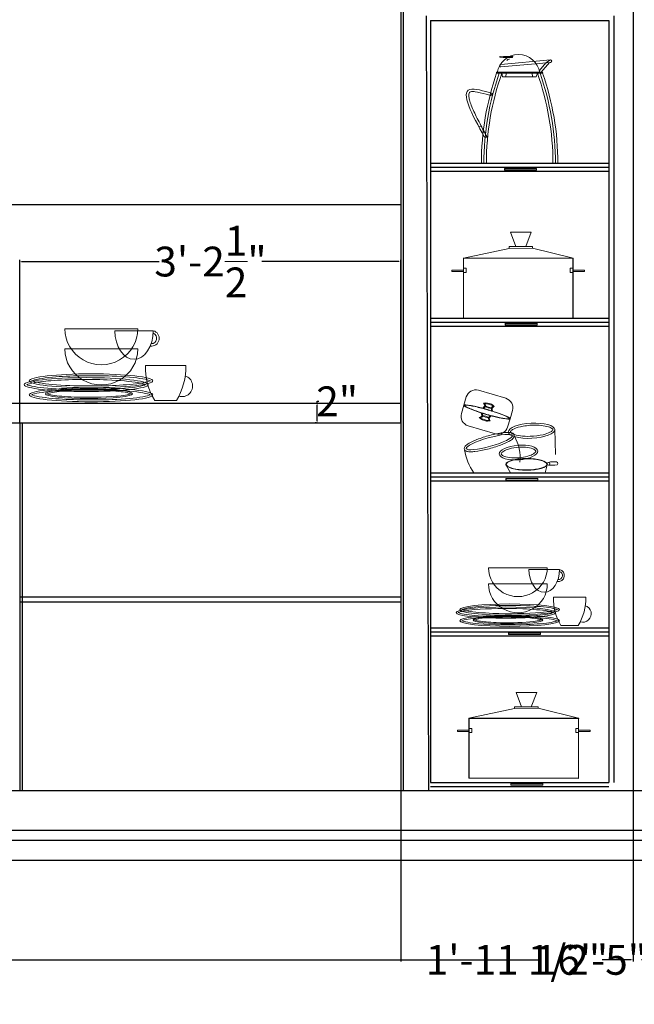
# Model space of a CAD drawing. Units: inches. Extents: x 1686244 to 1686928, y 1936095 to 1936489.
# Tile 3 of 11: x 1686303 to 1686365, y 1936336 to 1936435. Entities that reach past the tile are written whole.
import ezdxf

# ---------------------------------------------------------------- set-up
doc = ezdxf.new("R2010")
doc.units = ezdxf.units.IN
doc.header["$MEASUREMENT"] = 0
for name, color, linetype, lineweight in [('A-ANNO-DIMS', 240, 'Continuous', 18), ('A-ELEV', 7, 'Continuous', 25), ('A-FURN', 40, 'Continuous', 18)]:
    doc.layers.add(name, color=color, linetype=linetype, lineweight=lineweight)
doc.styles.get("Standard").update_dxf_attribs({"font": 'arial.ttf'})
doc.dimstyles.get("Standard").update_dxf_attribs({"dimtxt": 3, "dimasz": 0.18, "dimexe": 0.18, "dimexo": 0.0625, "dimgap": 0.09, "dimtad": 0, "dimtih": 1, "dimtoh": 1, "dimzin": 0, "dimdsep": 46, "dimlunit": 4, "dimtxsty": 'Standard', "dimcen": 0.09, "dimadec": 0, "dimazin": 0, "dimtfac": 1, "dimtofl": 0, "dimtmove": 0, "dimatfit": 3, "dimfxl": 1, "dimtolj": 1, "dimtzin": 0, "dimarcsym": 0})

# ---------------------------------------------------------------- blocks, each defined once
blk = doc.blocks.new('*D4')
at = {"layer": 'A-ANNO-DIMS', "color": 0, "lineweight": -2, "transparency": 16777216}
for p, q in [((1686303.305, 1936394.476), (1686303.305, 1936410.845)), ((1686303.485, 1936410.665), (1686317.355, 1936410.665)), ((1686341.513, 1936410.665), (1686327.696, 1936410.665)), ((1686341.693, 1936394.476), (1686341.693, 1936410.845))]:
    blk.add_line(p, q, dxfattribs=at)
at = {"layer": 'A-ANNO-DIMS', "color": 0, "transparency": 16777216}
for points in [[(1686303.485, 1936410.695), (1686303.485, 1936410.635), (1686303.305, 1936410.665)], [(1686341.513, 1936410.695), (1686341.513, 1936410.635), (1686341.693, 1936410.665)]]:
    blk.add_solid(points, dxfattribs=at)
at = {"layer": 'Defpoints', "color": 0, "transparency": 16777216}
for p in [(1686341.693, 1936410.665), (1686303.305, 1936394.414), (1686341.693, 1936394.414)]:
    blk.add_point(p, dxfattribs=at)
at = {"layer": 'A-ANNO-DIMS', "color": 0, "transparency": 16777216, "insert": (1686322.526, 1936410.665), "char_height": 3, "attachment_point": 5}
blk.add_mtext('\\A1;3\'-2{\\H1x;\\S1/2;}"', dxfattribs=at)
blk = doc.blocks.new('*D56')
at = {"layer": 'A-ANNO-DIMS', "color": 0, "lineweight": -2, "transparency": 16777216}
for p, q in [((1686333.27, 1936396.414), (1686333.27, 1936396.594)), ((1686333.27, 1936396.594), (1686333.45, 1936396.594)), ((1686333.27, 1936394.594), (1686333.27, 1936396.234)), ((1686333.333, 1936396.414), (1686333.45, 1936396.414)), ((1686333.208, 1936394.414), (1686333.09, 1936394.414))]:
    blk.add_line(p, q, dxfattribs=at)
at = {"layer": 'A-ANNO-DIMS', "color": 0, "transparency": 16777216}
for points in [[(1686333.24, 1936396.234), (1686333.3, 1936396.234), (1686333.27, 1936396.414)], [(1686333.24, 1936394.594), (1686333.3, 1936394.594), (1686333.27, 1936394.414)]]:
    blk.add_solid(points, dxfattribs=at)
at = {"layer": 'Defpoints', "color": 0, "transparency": 16777216}
for p in [(1686333.27, 1936396.414), (1686333.27, 1936396.414), (1686333.27, 1936394.414)]:
    blk.add_point(p, dxfattribs=at)
at = {"layer": 'A-ANNO-DIMS', "color": 0, "transparency": 16777216, "insert": (1686335.29, 1936396.594), "char_height": 3, "attachment_point": 5}
blk.add_mtext('\\A1;2"', dxfattribs=at)
blk = doc.blocks.new('COOKING-POT')
for p, q in [((0.009, 6.061), (4.609, 7.038)), ((4.609, 7.038), (4.609, 7.206)), ((4.609, 7.038), (6.983, 7.07)), ((4.629, 7.226), (6.962, 7.226)), ((6.982, 7.206), (6.983, 7.07)), ((11.059, 6.061), (6.983, 7.07)), ((0.029, 6.041), (0.009, 6.041)), ((11.039, 6.041), (11.059, 6.041))]:
    blk.add_line(p, q)
for points in [[(11.059, 6.061), (0.009, 6.061)], [(0.009, 0.022), (11.059, 0), (11.059, 6.041)], [(0.009, 6.041), (0.009, 0.022)]]:
    blk.add_lwpolyline(points)
blk.add_lwpolyline([(0.029, 0.042), (11.039, 0.022), (11.039, 6.041), (0.029, 6.041)], close=True)
for centre, radius, start, end in [((4.629, 7.206), 0.0201, 90, 180), ((6.962, 7.206), 0.0201, 0.77462, 90), ((0.01, 6.051), 0.0101, 93.59862, 266.40138), ((11.058, 6.051), 0.0101, 273.59862, 86.40138)]:
    blk.add_arc(centre, radius, start, end)
blk = doc.blocks.new('*D87')
at = {"layer": 'A-ANNO-DIMS', "color": 0, "lineweight": -2, "transparency": 16777216}
for p, q in [((1686262.353, 1936350.349), (1686262.353, 1936340.182)), ((1686459.353, 1936350.349), (1686459.353, 1936340.182)), ((1686262.533, 1936340.362), (1686355.751, 1936340.362)), ((1686459.173, 1936340.362), (1686365.954, 1936340.362))]:
    blk.add_line(p, q, dxfattribs=at)
at = {"layer": 'A-ANNO-DIMS', "color": 0, "transparency": 16777216}
for points in [[(1686262.533, 1936340.392), (1686262.533, 1936340.332), (1686262.353, 1936340.362)], [(1686459.173, 1936340.392), (1686459.173, 1936340.332), (1686459.353, 1936340.362)]]:
    blk.add_solid(points, dxfattribs=at)
at = {"layer": 'Defpoints', "color": 0, "transparency": 16777216}
for p in [(1686262.353, 1936350.412), (1686459.353, 1936350.412), (1686459.353, 1936340.362)]:
    blk.add_point(p, dxfattribs=at)
at = {"layer": 'A-ANNO-DIMS', "color": 0, "transparency": 16777216, "insert": (1686360.853, 1936340.362), "char_height": 3, "attachment_point": 5}
blk.add_mtext('\\A1;16\'-5"', dxfattribs=at)
blk = doc.blocks.new('*D90')
at = {"layer": 'A-ANNO-DIMS', "color": 0, "lineweight": -2, "transparency": 16777216}
for p, q in [((1686341.693, 1936357.349), (1686341.693, 1936340.182)), ((1686365.103, 1936357.349), (1686365.103, 1936340.182)), ((1686341.873, 1936340.362), (1686344.801, 1936340.362)), ((1686364.923, 1936340.362), (1686361.995, 1936340.362))]:
    blk.add_line(p, q, dxfattribs=at)
at = {"layer": 'A-ANNO-DIMS', "color": 0, "transparency": 16777216}
for points in [[(1686341.873, 1936340.392), (1686341.873, 1936340.332), (1686341.693, 1936340.362)], [(1686364.923, 1936340.392), (1686364.923, 1936340.332), (1686365.103, 1936340.362)]]:
    blk.add_solid(points, dxfattribs=at)
at = {"layer": 'Defpoints', "color": 0, "transparency": 16777216}
for p in [(1686341.693, 1936357.412), (1686365.103, 1936357.412), (1686365.103, 1936340.362)]:
    blk.add_point(p, dxfattribs=at)
at = {"layer": 'A-ANNO-DIMS', "color": 0, "transparency": 16777216, "insert": (1686353.398, 1936340.362), "char_height": 3, "attachment_point": 5}
blk.add_mtext('\\A1;1\'-11 1/2"', dxfattribs=at)

msp = doc.modelspace()

# ---------------------------------------------------------------- linework, layer by layer
at = {"layer": 'A-ELEV'}
for p, q in [((1686341.693, 1936467.412), (1686341.693, 1936357.412)), ((1686341.943, 1936467.412), (1686341.943, 1936357.412)), ((1686365.103, 1936467.412), (1686365.103, 1936357.412)), ((1686344.26, 1936435.412), (1686344.495, 1936357.412)), ((1686363.15, 1936435.412), (1686363.15, 1936358.215)), ((1686344.7, 1936434.948), (1686344.7, 1936358.215)), ((1686344.7, 1936434.948), (1686362.65, 1936434.948)), ((1686362.65, 1936434.948), (1686362.65, 1936358.215)), ((1686344.7, 1936420.566), (1686362.65, 1936420.566)), ((1686344.7, 1936420.164), (1686362.65, 1936420.164)), ((1686344.7, 1936419.762), (1686362.65, 1936419.762)), ((1686262.353, 1936416.412), (1686341.693, 1936416.412)), ((1686344.7, 1936404.978), (1686362.65, 1936404.978)), ((1686344.7, 1936404.576), (1686362.65, 1936404.576)), ((1686344.7, 1936404.175), (1686362.65, 1936404.175)), ((1686262.353, 1936396.412), (1686341.687, 1936396.414)), ((1686262.353, 1936394.412), (1686341.693, 1936394.414)), ((1686303.305, 1936394.414), (1686303.305, 1936357.414)), ((1686303.555, 1936394.414), (1686303.555, 1936357.414)), ((1686344.7, 1936389.391), (1686362.65, 1936389.391)), ((1686344.7, 1936388.989), (1686362.65, 1936388.989)), ((1686344.7, 1936388.587), (1686362.65, 1936388.587)), ((1686303.305, 1936376.914), (1686341.746, 1936376.914)), ((1686303.305, 1936376.414), (1686341.748, 1936376.414)), ((1686344.7, 1936373.803), (1686362.65, 1936373.803)), ((1686344.7, 1936373.401), (1686362.65, 1936373.401)), ((1686344.7, 1936372.999), (1686362.65, 1936372.999)), ((1686344.7, 1936358.215), (1686362.65, 1936358.215)), ((1686343.995, 1936357.412), (1686343.995, 1936357.41)), ((1686344.222, 1936357.412), (1686362.975, 1936357.412)), ((1686344.7, 1936357.814), (1686362.65, 1936357.814)), ((1686262.353, 1936353.412), (1686459.353, 1936353.412)), ((1686262.353, 1936352.412), (1686459.353, 1936352.412)), ((1686262.353, 1936350.412), (1686459.353, 1936350.412))]:
    msp.add_line(p, q, dxfattribs=at)
msp.add_lwpolyline([(1686459.353, 1936357.412), (1686459.353, 1936467.412), (1686262.353, 1936467.412), (1686262.353, 1936357.412)], close=True, dxfattribs=at)
at = {"layer": 'A-FURN'}
for p, q in [((1686351.713, 1936431.294), (1686352.069, 1936431.279)), ((1686352.084, 1936431.298), (1686352.011, 1936431.201)), ((1686352.992, 1936431.298), (1686352.084, 1936431.298)), ((1686352.969, 1936431.201), (1686352.992, 1936431.298)), ((1686352.048, 1936431.249), (1686351.685, 1936431.249)), ((1686351.763, 1936430.503), (1686356.77, 1936430.959)), ((1686351.786, 1936430.255), (1686356.793, 1936430.711)), ((1686352.011, 1936431.201), (1686352.969, 1936431.201)), ((1686356.327, 1936430.669), (1686355.661, 1936429.9)), ((1686356.684, 1936430.701), (1686355.831, 1936429.716)), ((1686356.782, 1936430.96), (1686356.327, 1936430.669)), ((1686351.359, 1936429.678), (1686351.359, 1936429.716)), ((1686351.359, 1936429.716), (1686355.991, 1936429.716)), ((1686351.359, 1936429.678), (1686355.991, 1936429.678)), ((1686351.359, 1936429.629), (1686355.991, 1936429.629)), ((1686351.886, 1936429.629), (1686351.955, 1936429.258)), ((1686352.328, 1936429.629), (1686352.277, 1936429.258)), ((1686354.895, 1936429.629), (1686355.006, 1936429.258)), ((1686355.331, 1936429.258), (1686355.464, 1936429.629)), ((1686355.991, 1936429.716), (1686355.991, 1936429.678)), ((1686351.955, 1936429.258), (1686355.331, 1936429.258)), ((1686350.957, 1936427.571), (1686350.765, 1936427.369)), ((1686349.549, 1936424.256), (1686349.803, 1936424.307)), ((1686350.408, 1936423.194), (1686350.127, 1936423.189)), ((1686349.821, 1936420.571), (1686357.528, 1936420.571)), ((1686349.821, 1936420.566), (1686357.528, 1936420.566)), ((1686353.3, 1936412.182), (1686352.753, 1936413.613)), ((1686352.753, 1936413.613), (1686354.833, 1936413.613)), ((1686354.286, 1936412.182), (1686354.833, 1936413.613)), ((1686348.007, 1936409.808), (1686346.848, 1936409.808)), ((1686346.848, 1936409.808), (1686346.848, 1936409.674)), ((1686346.848, 1936409.674), (1686348.007, 1936409.674)), ((1686348.007, 1936409.674), (1686348.007, 1936409.808)), ((1686359.057, 1936409.808), (1686360.216, 1936409.808)), ((1686359.057, 1936409.674), (1686359.057, 1936409.808)), ((1686360.216, 1936409.674), (1686359.057, 1936409.674)), ((1686360.216, 1936409.808), (1686360.216, 1936409.674)), ((1686307.855, 1936403.901), (1686315.213, 1936403.901)), ((1686312.902, 1936403.697), (1686316.76, 1936403.697)), ((1686307.855, 1936401.868), (1686315.213, 1936401.868)), ((1686315.975, 1936400.215), (1686320.037, 1936400.215)), ((1686316.918, 1936396.663), (1686319.094, 1936396.663)), ((1686357.217, 1936393.798), (1686357.274, 1936391.243)), ((1686352.366, 1936390.092), (1686352.754, 1936389.402)), ((1686356.251, 1936389.379), (1686356.451, 1936390.209)), ((1686352.754, 1936389.402), (1686356.251, 1936389.379)), ((1686350.548, 1936379.844), (1686356.46, 1936379.844)), ((1686354.603, 1936379.679), (1686357.703, 1936379.679)), ((1686350.548, 1936378.21), (1686356.46, 1936378.21)), ((1686357.072, 1936376.882), (1686360.336, 1936376.882)), ((1686357.83, 1936374.028), (1686359.578, 1936374.028)), ((1686353.862, 1936365.849), (1686353.315, 1936367.281)), ((1686353.315, 1936367.281), (1686355.395, 1936367.281)), ((1686354.848, 1936365.849), (1686355.395, 1936367.281)), ((1686348.569, 1936363.476), (1686347.41, 1936363.476)), ((1686347.41, 1936363.476), (1686347.41, 1936363.342)), ((1686347.41, 1936363.342), (1686348.569, 1936363.342)), ((1686348.569, 1936363.342), (1686348.569, 1936363.476)), ((1686359.619, 1936363.476), (1686360.778, 1936363.476)), ((1686359.619, 1936363.342), (1686359.619, 1936363.476)), ((1686360.778, 1936363.342), (1686359.619, 1936363.342)), ((1686360.778, 1936363.476), (1686360.778, 1936363.342))]:
    msp.add_line(p, q, dxfattribs=at)
for points in [[(1686352.147, 1936420.033), (1686355.381, 1936420.034), (1686355.381, 1936419.857), (1686352.147, 1936419.855)], [(1686352.167, 1936420.013), (1686355.361, 1936420.014), (1686355.361, 1936419.877), (1686352.167, 1936419.875)], [(1686348.3, 1936409.992), (1686348.027, 1936409.992), (1686348.027, 1936409.569), (1686348.3, 1936409.569)], [(1686358.764, 1936409.992), (1686359.037, 1936409.992), (1686359.037, 1936409.569), (1686358.764, 1936409.569)], [(1686352.219, 1936404.452), (1686355.454, 1936404.454), (1686355.454, 1936404.276), (1686352.219, 1936404.275)], [(1686352.239, 1936404.432), (1686355.434, 1936404.434), (1686355.434, 1936404.296), (1686352.239, 1936404.295)], [(1686352.29, 1936388.829), (1686355.524, 1936388.83), (1686355.524, 1936388.653), (1686352.29, 1936388.651)], [(1686352.31, 1936388.809), (1686355.504, 1936388.81), (1686355.504, 1936388.673), (1686352.31, 1936388.672)], [(1686352.553, 1936373.301), (1686355.787, 1936373.303), (1686355.787, 1936373.125), (1686352.553, 1936373.124)], [(1686352.573, 1936373.281), (1686355.767, 1936373.282), (1686355.767, 1936373.145), (1686352.573, 1936373.144)], [(1686348.862, 1936363.659), (1686348.589, 1936363.659), (1686348.589, 1936363.237), (1686348.862, 1936363.237)], [(1686359.326, 1936363.659), (1686359.599, 1936363.659), (1686359.599, 1936363.237), (1686359.326, 1936363.237)], [(1686352.781, 1936358.12), (1686356.016, 1936358.121), (1686356.016, 1936357.944), (1686352.781, 1936357.942)], [(1686352.801, 1936358.1), (1686355.996, 1936358.101), (1686355.996, 1936357.964), (1686352.801, 1936357.962)]]:
    msp.add_lwpolyline(points, close=True, dxfattribs=at)
for points in [[(1686348.054, 1936396.197), (1686348.3, 1936397.036, -0.414214), (1686349.522, 1936397.705), (1686352.284, 1936396.896, -0.414214), (1686352.953, 1936395.674), (1686352.707, 1936394.835)], [(1686348.054, 1936396.197), (1686347.808, 1936395.358, 0.414214), (1686348.477, 1936394.136), (1686351.239, 1936393.327, 0.414214), (1686352.462, 1936393.996), (1686352.707, 1936394.835)]]:
    msp.add_lwpolyline(points, format="xyb", dxfattribs=at)
for centre, radius, start, end in [((1686353.561, 1936429.323), 2.177, 9.38599, 170.61401), ((1686351.701, 1936431.27), 0.0262, 61.61926, 233.31707), ((1686351.775, 1936430.379), 0.124, 95.20713, 275.20713), ((1686352.619, 1936430.803), 0.24, 80.65216, 158.47241), ((1686356.782, 1936430.835), 0.124, 275.20713, 95.20713), ((1686377.643, 1936420.509), 27.821, 160.8647, 179.88296), ((1686377.643, 1936420.509), 27.572, 160.68521, 179.88296), ((1686377.643, 1936420.509), 27.324, 160.50225, 179.88296), ((1686351.359, 1936429.654), 0.0249, 90, 270), ((1686329.707, 1936420.509), 27.324, 0.11704, 19.49775), ((1686329.707, 1936420.509), 27.572, 0.11704, 19.31479), ((1686355.991, 1936429.654), 0.0249, 270, 90), ((1686329.707, 1936420.509), 27.821, 0.11704, 19.1353), ((1686316.58, 1936402.935), 0.783, 261.33254, 76.68363), ((1686316.58, 1936402.935), 0.533, 267.18688, 71.10649), ((1686322.385, 1936400.015), 6.413, 178.21878, 211.51741), ((1686313.627, 1936400.015), 6.413, 328.48259, 1.78122), ((1686319.669, 1936398.129), 1.059, 252.39211, 72.93123), ((1686351.263, 1936398.46), 2.63, 246.06969, 260.59906), ((1686351.263, 1936398.46), 2.553, 246.09715, 260.54093), ((1686349.536, 1936392.561), 2.553, 66.8207, 81.26447), ((1686349.536, 1936392.561), 2.63, 66.76257, 81.29193), ((1686349.351, 1936390.932), 4.367, 353.73815, 29.7733), ((1686353.531, 1936392.564), 5.47, 188.81379, 215.45739), ((1686357.558, 1936379.067), 0.629, 261.33254, 76.68363), ((1686357.558, 1936379.067), 0.428, 267.18688, 71.10649), ((1686362.222, 1936376.721), 5.153, 178.21878, 211.51741), ((1686355.186, 1936376.721), 5.153, 328.48259, 1.78122), ((1686360.04, 1936375.206), 0.851, 252.39211, 72.93123)]:
    msp.add_arc(centre, radius, start, end, dxfattribs=at)
for centre, major_axis, ratio, start_param, end_param in [((1686311.534, 1936403.901), (-3.679, 0), 0.984479, 0, 3.141593), ((1686314.831, 1936403.697), (0, -2.875), 0.670965, -1.570796, 1.570796), ((1686311.534, 1936401.868), (-3.679, 0), 0.984479, 0, 3.141593), ((1686356.588, 1936390.302), (0, 0.145), 0.973714, -3.141592653589793, 3.141592653589793), ((1686353.504, 1936379.844), (-2.956, 0), 0.984479, 0, 3.141593), ((1686356.153, 1936379.679), (0, -2.31), 0.670965, -1.570796, 1.570796), ((1686353.504, 1936378.21), (-2.956, 0), 0.984479, 0, 3.141593)]:
    msp.add_ellipse(centre, major_axis=major_axis, ratio=ratio, start_param=start_param, end_param=end_param, dxfattribs=at)
for centre, major_axis, ratio in [((1686310.005, 1936398.275), (-6.238, 0), 0.112716), ((1686310.496, 1936398.658), (-6.238, 0), 0.112716), ((1686310.283, 1936397.361), (-4.385, 0), 0.112716), ((1686350.381, 1936395.516), (-2.327, 0.681), 0.103756), ((1686354.88, 1936393.632), (-2.343, -0.123), 0.322421), ((1686350.62, 1936392.49), (-2.316, -0.658), 0.180882), ((1686353.56, 1936391.436), (-1.938, -0.16), 0.37765), ((1686354.373, 1936390.249), (-2.083, 0), 0.283655), ((1686352.276, 1936375.323), (-5.012, 0), 0.112716), ((1686352.67, 1936375.631), (-5.012, 0), 0.112716), ((1686352.499, 1936374.589), (-3.523, 0), 0.112716)]:
    msp.add_ellipse(centre, major_axis=major_axis, ratio=ratio, dxfattribs=at)
at = {"layer": 'A-FURN', "extrusion": (0, 0, -1)}
for centre, major_axis in [((1686310.496, 1936397.251), (-6.238, 0)), ((1686352.67, 1936374.501), (-5.012, 0))]:
    msp.add_ellipse(centre, major_axis=major_axis, ratio=0.112716, dxfattribs=at)
at = {"layer": 'A-FURN'}
for points, knots in [([(1686350.957, 1936427.571), (1686350.031, 1936427.853), (1686347.119, 1936428.732), (1686348.884, 1936425.458), (1686350.127, 1936423.189)], [0.025615, 0.025615, 0.025615, 0.025615, 2.381971, 7.473739, 7.473739, 7.473739, 7.473739]), ([(1686350.765, 1936427.369), (1686350.605, 1936427.418), (1686350.445, 1936427.466), (1686349.883, 1936427.629), (1686349.501, 1936427.725), (1686349.057, 1936427.781), (1686348.931, 1936427.785), (1686348.744, 1936427.766), (1686348.689, 1936427.745), (1686348.62, 1936427.698), (1686348.599, 1936427.673), (1686348.56, 1936427.575), (1686348.546, 1936427.501), (1686348.548, 1936427.305), (1686348.564, 1936427.185), (1686348.662, 1936426.744), (1686348.803, 1936426.36), (1686349.183, 1936425.504), (1686349.421, 1936425.03), (1686349.912, 1936424.099), (1686350.16, 1936423.647), (1686350.408, 1936423.194)], [0.126779, 0.126779, 0.126779, 0.126779, 0.537653, 0.537653, 1.612958, 1.612958, 2.136642, 2.136642, 2.660327, 2.660327, 3.184011, 3.184011, 3.707696, 3.707696, 4.23138, 4.23138, 5.387407, 5.387407, 6.543433, 6.543433, 7.559303, 7.559303, 7.559303, 7.559303]), ([(1686315.992, 1936398.275), (1686315.859, 1936398.337), (1686315.588, 1936398.412), (1686314.5, 1936398.602), (1686313.393, 1936398.702), (1686310.139, 1936398.835), (1686307.783, 1936398.792), (1686305.066, 1936398.548), (1686304.28, 1936398.397), (1686304.018, 1936398.275)], [3.378504, 3.378504, 3.378504, 3.378504, 3.713925, 3.713925, 4.364024, 4.364024, 5.385398, 5.385398, 6.046274, 6.046274, 6.046274, 6.046274]), ([(1686316.483, 1936398.658), (1686316.35, 1936398.72), (1686316.079, 1936398.794), (1686314.991, 1936398.985), (1686313.884, 1936399.085), (1686310.63, 1936399.218), (1686308.273, 1936399.174), (1686305.557, 1936398.93), (1686304.771, 1936398.78), (1686304.509, 1936398.658)], [3.378504, 3.378504, 3.378504, 3.378504, 3.713925, 3.713925, 4.364024, 4.364024, 5.385398, 5.385398, 6.046274, 6.046274, 6.046274, 6.046274]), ([(1686304.509, 1936398.658), (1686304.642, 1936398.596), (1686304.913, 1936398.521), (1686306.001, 1936398.331), (1686307.108, 1936398.231), (1686310.362, 1936398.097), (1686312.719, 1936398.141), (1686315.435, 1936398.385), (1686316.221, 1936398.536), (1686316.483, 1936398.658)], [0.236911, 0.236911, 0.236911, 0.236911, 0.572332, 0.572332, 1.222431, 1.222431, 2.243805, 2.243805, 2.904681, 2.904681, 2.904681, 2.904681]), ([(1686304.018, 1936398.275), (1686304.151, 1936398.213), (1686304.422, 1936398.138), (1686305.51, 1936397.948), (1686306.618, 1936397.848), (1686309.872, 1936397.715), (1686312.228, 1936397.758), (1686314.945, 1936398.002), (1686315.731, 1936398.153), (1686315.992, 1936398.275)], [0.236911, 0.236911, 0.236911, 0.236911, 0.572332, 0.572332, 1.222431, 1.222431, 2.243805, 2.243805, 2.904681, 2.904681, 2.904681, 2.904681]), ([(1686304.509, 1936397.251), (1686304.642, 1936397.313), (1686304.913, 1936397.388), (1686306.001, 1936397.578), (1686307.108, 1936397.679), (1686310.362, 1936397.812), (1686312.719, 1936397.768), (1686315.435, 1936397.524), (1686316.221, 1936397.373), (1686316.483, 1936397.251)], [0.236911, 0.236911, 0.236911, 0.236911, 0.572332, 0.572332, 1.222431, 1.222431, 2.243805, 2.243805, 2.904681, 2.904681, 2.904681, 2.904681]), ([(1686314.491, 1936397.361), (1686314.398, 1936397.404), (1686314.208, 1936397.457), (1686313.443, 1936397.59), (1686312.664, 1936397.661), (1686310.377, 1936397.754), (1686308.721, 1936397.724), (1686306.812, 1936397.552), (1686306.259, 1936397.446), (1686306.075, 1936397.361)], [3.378504, 3.378504, 3.378504, 3.378504, 3.713925, 3.713925, 4.364024, 4.364024, 5.385398, 5.385398, 6.046274, 6.046274, 6.046274, 6.046274]), ([(1686316.483, 1936397.251), (1686316.35, 1936397.189), (1686316.079, 1936397.115), (1686314.991, 1936396.924), (1686313.884, 1936396.824), (1686310.63, 1936396.691), (1686308.273, 1936396.735), (1686305.557, 1936396.979), (1686304.771, 1936397.129), (1686304.509, 1936397.251)], [3.378504, 3.378504, 3.378504, 3.378504, 3.713925, 3.713925, 4.364024, 4.364024, 5.385398, 5.385398, 6.046274, 6.046274, 6.046274, 6.046274]), ([(1686306.075, 1936397.361), (1686306.169, 1936397.317), (1686306.359, 1936397.264), (1686307.124, 1936397.131), (1686307.902, 1936397.06), (1686310.189, 1936396.967), (1686311.846, 1936396.997), (1686313.755, 1936397.169), (1686314.308, 1936397.275), (1686314.491, 1936397.361)], [0.236911, 0.236911, 0.236911, 0.236911, 0.572332, 0.572332, 1.222431, 1.222431, 2.243805, 2.243805, 2.904681, 2.904681, 2.904681, 2.904681]), ([(1686348.077, 1936396.19), (1686348.077, 1936396.19), (1686348.077, 1936396.185), (1686348.092, 1936396.163), (1686348.107, 1936396.148), (1686348.179, 1936396.093), (1686348.264, 1936396.044), (1686348.627, 1936395.868), (1686349.017, 1936395.717), (1686349.927, 1936395.409), (1686350.446, 1936395.254), (1686351.314, 1936395.027), (1686351.676, 1936394.944), (1686352.258, 1936394.836), (1686352.479, 1936394.812), (1686352.638, 1936394.821), (1686352.667, 1936394.829), (1686352.685, 1936394.84), (1686352.684, 1936394.841), (1686352.684, 1936394.844), (1686352.682, 1936394.852), (1686352.663, 1936394.875), (1686352.647, 1936394.89), (1686352.567, 1936394.949), (1686352.468, 1936395.004), (1686352.094, 1936395.179), (1686351.738, 1936395.316), (1686350.913, 1936395.597), (1686350.446, 1936395.739), (1686349.547, 1936395.982), (1686349.118, 1936396.083), (1686348.45, 1936396.206), (1686348.209, 1936396.226), (1686348.095, 1936396.203), (1686348.082, 1936396.196), (1686348.077, 1936396.191), (1686348.077, 1936396.191), (1686348.077, 1936396.19)], [0, 0, 0, 0, 0.129873, 0.129873, 0.259747, 0.259747, 0.557497, 0.557497, 1.196564, 1.196564, 1.835631, 1.835631, 2.348435, 2.348435, 2.861238, 2.861238, 3.048242, 3.048242, 3.170903, 3.170903, 3.293565, 3.293565, 3.416226, 3.416226, 3.737883, 3.737883, 4.321058, 4.321058, 4.904233, 4.904233, 5.496223, 5.496223, 6.088213, 6.088213, 6.228874, 6.228874, 6.283185, 6.283185, 6.283185, 6.283185]), ([(1686349.96, 1936395.895), (1686350.082, 1936396.021), (1686350.156, 1936396.121), (1686350.165, 1936396.206), (1686350.158, 1936396.226), (1686350.117, 1936396.285), (1686350.1, 1936396.306), (1686350.03, 1936396.409)], [0, 0, 0, 0, 0.1303544, 0.1303544, 0.1938501, 0.1938501, 0.2257011, 0.2257011, 0.2257011, 0.2257011]), ([(1686350.03, 1936396.409), (1686350.348, 1936396.462), (1686350.558, 1936396.405), (1686350.868, 1936396.295), (1686350.98, 1936396.228), (1686351.118, 1936396.076)], [0, 0, 0, 0, 0.2296311, 0.2296311, 0.3676138, 0.3676138, 0.3676138, 0.3676138]), ([(1686350.052, 1936395.87), (1686350.159, 1936395.993), (1686350.312, 1936396.168), (1686350.18, 1936396.329), (1686350.141, 1936396.377)], [0, 0, 0, 0, 0.4052635, 0.5775496, 0.5775496, 0.5775496, 0.5775496]), ([(1686350.141, 1936396.377), (1686350.419, 1936396.344), (1686350.741, 1936396.304), (1686350.997, 1936396.122), (1686351.032, 1936396.097)], [0, 0, 0, 0, 0.812223, 0.9406919, 0.9406919, 0.9406919, 0.9406919]), ([(1686350.87, 1936395.637), (1686350.834, 1936395.785), (1686350.792, 1936395.994), (1686350.974, 1936396.073), (1686351.031, 1936396.098)], [0.0103618, 0.0103618, 0.0103618, 0.0103618, 0.1583733, 0.2257011, 0.2257011, 0.2257011, 0.2257011]), ([(1686350.957, 1936395.612), (1686350.92, 1936395.759), (1686350.903, 1936395.855), (1686350.922, 1936395.945), (1686350.932, 1936395.96), (1686350.993, 1936395.997), (1686351.026, 1936396.012), (1686351.118, 1936396.076)], [0.0103618, 0.0103618, 0.0103618, 0.0103618, 0.1154664, 0.1154664, 0.1835905, 0.1835905, 0.2257011, 0.2257011, 0.2257011, 0.2257011]), ([(1686349.822, 1936395.424), (1686349.857, 1936395.251), (1686349.866, 1936395.128), (1686349.827, 1936395.052), (1686349.81, 1936395.038), (1686349.744, 1936395.011), (1686349.718, 1936395.002), (1686349.604, 1936394.953)], [0, 0, 0, 0, 0.1303544, 0.1303544, 0.1938501, 0.1938501, 0.2257011, 0.2257011, 0.2257011, 0.2257011]), ([(1686349.604, 1936394.953), (1686349.843, 1936394.737), (1686350.05, 1936394.672), (1686350.371, 1936394.598), (1686350.502, 1936394.593), (1686350.699, 1936394.646)], [0, 0, 0, 0, 0.2296311, 0.2296311, 0.3676138, 0.3676138, 0.3676138, 0.3676138]), ([(1686349.913, 1936395.395), (1686349.937, 1936395.234), (1686349.971, 1936395.004), (1686349.773, 1936394.939), (1686349.714, 1936394.92)], [0, 0, 0, 0, 0.4052635, 0.5775496, 0.5775496, 0.5775496, 0.5775496]), ([(1686349.714, 1936394.92), (1686349.966, 1936394.799), (1686350.259, 1936394.658), (1686350.573, 1936394.673), (1686350.616, 1936394.675)], [0, 0, 0, 0, 0.812223, 0.9406919, 0.9406919, 0.9406919, 0.9406919]), ([(1686350.728, 1936395.15), (1686350.618, 1936395.045), (1686350.469, 1936394.891), (1686350.58, 1936394.727), (1686350.615, 1936394.675)], [0.0103618, 0.0103618, 0.0103618, 0.0103618, 0.1583733, 0.2257011, 0.2257011, 0.2257011, 0.2257011]), ([(1686350.814, 1936395.125), (1686350.704, 1936395.021), (1686350.638, 1936394.948), (1686350.606, 1936394.863), (1686350.606, 1936394.845), (1686350.637, 1936394.78), (1686350.657, 1936394.75), (1686350.699, 1936394.646)], [0.0103618, 0.0103618, 0.0103618, 0.0103618, 0.1154664, 0.1154664, 0.1835905, 0.1835905, 0.2257011, 0.2257011, 0.2257011, 0.2257011]), ([(1686352.738, 1936393.519), (1686352.738, 1936393.511), (1686352.74, 1936393.5), (1686352.769, 1936393.458), (1686352.796, 1936393.429), (1686352.885, 1936393.365), (1686352.946, 1936393.332), (1686353.196, 1936393.224), (1686353.45, 1936393.159), (1686354.045, 1936393.077), (1686354.386, 1936393.06), (1686355.186, 1936393.082), (1686355.647, 1936393.141), (1686356.316, 1936393.301), (1686356.558, 1936393.388), (1686356.84, 1936393.536), (1686356.92, 1936393.595), (1686357, 1936393.68), (1686357.014, 1936393.708), (1686357.025, 1936393.741), (1686357.024, 1936393.745), (1686357.016, 1936393.771), (1686357.003, 1936393.794), (1686356.939, 1936393.855), (1686356.889, 1936393.891), (1686356.688, 1936393.995), (1686356.489, 1936394.06), (1686356.006, 1936394.154), (1686355.723, 1936394.184), (1686354.96, 1936394.208), (1686354.457, 1936394.171), (1686353.669, 1936394.028), (1686353.359, 1936393.938), (1686353, 1936393.776), (1686352.895, 1936393.711), (1686352.782, 1936393.612), (1686352.756, 1936393.575), (1686352.738, 1936393.535), (1686352.737, 1936393.527), (1686352.738, 1936393.519)], [0, 0, 0, 0, 0.193033, 0.193033, 0.386066, 0.386066, 0.579098, 0.579098, 1.036223, 1.036223, 1.493347, 1.493347, 2.091015, 2.091015, 2.531383, 2.531383, 2.814347, 2.814347, 3.022047, 3.022047, 3.229746, 3.229746, 3.437445, 3.437445, 3.645144, 3.645144, 4.05192, 4.05192, 4.458696, 4.458696, 5.088556, 5.088556, 5.589787, 5.589787, 5.892877, 5.892877, 6.117294, 6.117294, 6.283185, 6.283185, 6.283185, 6.283185]), ([(1686348.111, 1936391.778), (1686348.126, 1936391.726), (1686348.157, 1936391.68), (1686348.225, 1936391.615), (1686348.262, 1936391.593), (1686348.335, 1936391.56), (1686348.373, 1936391.548), (1686348.508, 1936391.517), (1686348.617, 1936391.509), (1686348.871, 1936391.511), (1686349.016, 1936391.521), (1686349.536, 1936391.58), (1686349.974, 1936391.665), (1686350.88, 1936391.895), (1686351.345, 1936392.039), (1686352.079, 1936392.314), (1686352.367, 1936392.441), (1686352.716, 1936392.63), (1686352.821, 1936392.696), (1686352.97, 1936392.811), (1686353.022, 1936392.86), (1686353.093, 1936392.957), (1686353.118, 1936393), (1686353.142, 1936393.1), (1686353.143, 1936393.154), (1686353.113, 1936393.257), (1686353.083, 1936393.301), (1686353.016, 1936393.365), (1686352.98, 1936393.387), (1686352.909, 1936393.419), (1686352.872, 1936393.431), (1686352.739, 1936393.463), (1686352.633, 1936393.471), (1686352.384, 1936393.471), (1686352.242, 1936393.462), (1686351.732, 1936393.405), (1686351.301, 1936393.323), (1686350.407, 1936393.1), (1686349.946, 1936392.959), (1686349.2, 1936392.684), (1686348.9, 1936392.554), (1686348.538, 1936392.36), (1686348.43, 1936392.293), (1686348.277, 1936392.176), (1686348.223, 1936392.127), (1686348.15, 1936392.03), (1686348.124, 1936391.987), (1686348.098, 1936391.886), (1686348.096, 1936391.831), (1686348.111, 1936391.778)], [0, 0, 0, 0, 0.105893, 0.105893, 0.211786, 0.211786, 0.317679, 0.317679, 0.576196, 0.576196, 0.834713, 0.834713, 1.414893, 1.414893, 1.995073, 1.995073, 2.461973, 2.461973, 2.72225, 2.72225, 2.914346, 2.914346, 3.039937, 3.039937, 3.143354, 3.143354, 3.246771, 3.246771, 3.350188, 3.350188, 3.453605, 3.453605, 3.709337, 3.709337, 3.965069, 3.965069, 4.5386, 4.5386, 5.112131, 5.112131, 5.590821, 5.590821, 5.854021, 5.854021, 6.049742, 6.049742, 6.177036, 6.177036, 6.283185, 6.283185, 6.283185, 6.283185]), ([(1686351.821, 1936391.293), (1686351.823, 1936391.278), (1686351.827, 1936391.262), (1686351.862, 1936391.212), (1686351.894, 1936391.181), (1686351.99, 1936391.115), (1686352.055, 1936391.081), (1686352.318, 1936390.978), (1686352.58, 1936390.923), (1686353.172, 1936390.877), (1686353.502, 1936390.887), (1686354.135, 1936390.967), (1686354.438, 1936391.038), (1686354.882, 1936391.201), (1686355.042, 1936391.287), (1686355.214, 1936391.421), (1686355.258, 1936391.472), (1686355.295, 1936391.54), (1686355.298, 1936391.56), (1686355.298, 1936391.59), (1686355.294, 1936391.605), (1686355.262, 1936391.654), (1686355.232, 1936391.686), (1686355.136, 1936391.754), (1686355.07, 1936391.789), (1686354.808, 1936391.893), (1686354.549, 1936391.948), (1686353.964, 1936391.995), (1686353.637, 1936391.987), (1686353.007, 1936391.91), (1686352.705, 1936391.84), (1686352.253, 1936391.679), (1686352.087, 1936391.592), (1686351.909, 1936391.455), (1686351.864, 1936391.404), (1686351.823, 1936391.33), (1686351.82, 1936391.31), (1686351.821, 1936391.293)], [0, 0, 0, 0, 0.218372, 0.218372, 0.436745, 0.436745, 0.655117, 0.655117, 1.170938, 1.170938, 1.686759, 1.686759, 2.20258, 2.20258, 2.618678, 2.618678, 2.894855, 2.894855, 3.119413, 3.119413, 3.343972, 3.343972, 3.56853, 3.56853, 3.793089, 3.793089, 4.304895, 4.304895, 4.816702, 4.816702, 5.328508, 5.328508, 5.75235, 5.75235, 6.030072, 6.030072, 6.283185, 6.283185, 6.283185, 6.283185]), ([(1686352.323, 1936390.249), (1686352.323, 1936390.198), (1686352.353, 1936390.143), (1686352.487, 1936390.029), (1686352.59, 1936389.973), (1686353.023, 1936389.81), (1686353.478, 1936389.729), (1686354.467, 1936389.674), (1686354.997, 1936389.7), (1686355.781, 1936389.832), (1686356.068, 1936389.922), (1686356.346, 1936390.088), (1686356.405, 1936390.156), (1686356.434, 1936390.276), (1686356.411, 1936390.337), (1686356.265, 1936390.468), (1686356.143, 1936390.533), (1686355.668, 1936390.7), (1686355.201, 1936390.777), (1686354.202, 1936390.823), (1686353.674, 1936390.791), (1686352.918, 1936390.653), (1686352.65, 1936390.564), (1686352.395, 1936390.403), (1686352.341, 1936390.339), (1686352.324, 1936390.27), (1686352.323, 1936390.26), (1686352.323, 1936390.249)], [0, 0, 0, 0, 0.323549, 0.323549, 0.647097, 0.647097, 1.376352, 1.376352, 2.105606, 2.105606, 2.698637, 2.698637, 3.072846, 3.072846, 3.447055, 3.447055, 3.821265, 3.821265, 4.553416, 4.553416, 5.285566, 5.285566, 5.858503, 5.858503, 6.21544, 6.21544, 6.283185, 6.283185, 6.283185, 6.283185]), ([(1686356.578, 1936390.447), (1686356.706, 1936390.492), (1686356.911, 1936390.493), (1686357.186, 1936390.487), (1686357.328, 1936390.501), (1686357.397, 1936390.51)], [0, 0, 0, 0, 0.916458, 1.428142, 1.911036, 1.911036, 1.911036, 1.911036]), ([(1686357.397, 1936390.51), (1686357.466, 1936390.459), (1686357.533, 1936390.358), (1686357.49, 1936390.242), (1686357.444, 1936390.185)], [0.0418453, 0.0418453, 0.0418453, 0.0418453, 0.5382692, 0.9735226, 0.9735226, 0.9735226, 0.9735226]), ([(1686357.086, 1936375.323), (1686356.979, 1936375.373), (1686356.761, 1936375.433), (1686355.887, 1936375.586), (1686354.998, 1936375.666), (1686352.383, 1936375.773), (1686350.49, 1936375.738), (1686348.307, 1936375.542), (1686347.675, 1936375.421), (1686347.465, 1936375.323)], [3.378504, 3.378504, 3.378504, 3.378504, 3.713925, 3.713925, 4.364024, 4.364024, 5.385398, 5.385398, 6.046274, 6.046274, 6.046274, 6.046274]), ([(1686357.48, 1936375.631), (1686357.374, 1936375.681), (1686357.156, 1936375.741), (1686356.282, 1936375.893), (1686355.392, 1936375.974), (1686352.777, 1936376.081), (1686350.884, 1936376.046), (1686348.701, 1936375.85), (1686348.07, 1936375.729), (1686347.86, 1936375.631)], [3.378504, 3.378504, 3.378504, 3.378504, 3.713925, 3.713925, 4.364024, 4.364024, 5.385398, 5.385398, 6.046274, 6.046274, 6.046274, 6.046274]), ([(1686347.465, 1936375.323), (1686347.572, 1936375.273), (1686347.79, 1936375.213), (1686348.664, 1936375.061), (1686349.554, 1936374.98), (1686352.168, 1936374.873), (1686354.062, 1936374.908), (1686356.244, 1936375.104), (1686356.876, 1936375.225), (1686357.086, 1936375.323)], [0.236911, 0.236911, 0.236911, 0.236911, 0.572332, 0.572332, 1.222431, 1.222431, 2.243805, 2.243805, 2.904681, 2.904681, 2.904681, 2.904681]), ([(1686347.86, 1936375.631), (1686347.966, 1936375.581), (1686348.184, 1936375.521), (1686349.058, 1936375.368), (1686349.948, 1936375.288), (1686352.563, 1936375.181), (1686354.456, 1936375.216), (1686356.639, 1936375.412), (1686357.27, 1936375.533), (1686357.48, 1936375.631)], [0.236911, 0.236911, 0.236911, 0.236911, 0.572332, 0.572332, 1.222431, 1.222431, 2.243805, 2.243805, 2.904681, 2.904681, 2.904681, 2.904681]), ([(1686347.86, 1936374.501), (1686347.966, 1936374.551), (1686348.184, 1936374.611), (1686349.058, 1936374.764), (1686349.948, 1936374.844), (1686352.563, 1936374.951), (1686354.456, 1936374.916), (1686356.639, 1936374.72), (1686357.27, 1936374.599), (1686357.48, 1936374.501)], [0.236911, 0.236911, 0.236911, 0.236911, 0.572332, 0.572332, 1.222431, 1.222431, 2.243805, 2.243805, 2.904681, 2.904681, 2.904681, 2.904681]), ([(1686355.88, 1936374.589), (1686355.805, 1936374.623), (1686355.652, 1936374.666), (1686355.038, 1936374.773), (1686354.412, 1936374.83), (1686352.575, 1936374.905), (1686351.244, 1936374.88), (1686349.71, 1936374.742), (1686349.266, 1936374.657), (1686349.118, 1936374.589)], [3.378504, 3.378504, 3.378504, 3.378504, 3.713925, 3.713925, 4.364024, 4.364024, 5.385398, 5.385398, 6.046274, 6.046274, 6.046274, 6.046274]), ([(1686357.48, 1936374.501), (1686357.374, 1936374.451), (1686357.156, 1936374.391), (1686356.282, 1936374.238), (1686355.392, 1936374.158), (1686352.777, 1936374.051), (1686350.884, 1936374.086), (1686348.701, 1936374.282), (1686348.07, 1936374.403), (1686347.86, 1936374.501)], [3.378504, 3.378504, 3.378504, 3.378504, 3.713925, 3.713925, 4.364024, 4.364024, 5.385398, 5.385398, 6.046274, 6.046274, 6.046274, 6.046274]), ([(1686349.118, 1936374.589), (1686349.193, 1936374.554), (1686349.346, 1936374.511), (1686349.961, 1936374.404), (1686350.586, 1936374.347), (1686352.424, 1936374.272), (1686353.754, 1936374.297), (1686355.289, 1936374.435), (1686355.733, 1936374.52), (1686355.88, 1936374.589)], [0.236911, 0.236911, 0.236911, 0.236911, 0.572332, 0.572332, 1.222431, 1.222431, 2.243805, 2.243805, 2.904681, 2.904681, 2.904681, 2.904681])]:
    msp.add_open_spline(points, degree=3, knots=knots, dxfattribs=at)
msp.add_open_spline([(1686356.579, 1936390.157), (1686356.867, 1936390.171), (1686357.156, 1936390.185), (1686357.444, 1936390.185)], degree=3, dxfattribs=at)

# ---------------------------------------------------------------- block references
for p in [(1686347.998, 1936404.956), (1686348.56, 1936358.623)]:
    msp.add_blockref('COOKING-POT', p, dxfattribs=at)

# ---------------------------------------------------------------- dimensions: what is measured, and where the dimension line sits
at = {"layer": 'A-ANNO-DIMS'}
dim = msp.add_linear_dim(base=(1686341.693, 1936410.665), p1=(1686303.305, 1936394.414), p2=(1686341.693, 1936394.414), dimstyle='Standard', override={"dimclrd": 0, "dimclre": 0, "dimclrt": 0}, dxfattribs=at)
dim.commit()
dim.dimension.update_dxf_attribs({"geometry": '*D4', "text_midpoint": (1686322.526, 1936410.665), "dimtype": 160})
dim = msp.add_linear_dim(base=(1686333.27, 1936396.414), p1=(1686333.27, 1936394.414), p2=(1686333.27, 1936396.414), angle=90, dimstyle='Standard', override={"dimclrd": 0, "dimclre": 0, "dimclrt": 0}, dxfattribs=at)
dim.commit()
dim.dimension.update_dxf_attribs({"geometry": '*D56', "text_midpoint": (1686335.29, 1936396.594)})
for base, p1, p2, picture, middle in [((1686365.103, 1936340.362), (1686341.693, 1936357.412), (1686365.103, 1936357.412), '*D90', (1686353.398, 1936340.362)), ((1686459.353, 1936340.362), (1686262.353, 1936350.412), (1686459.353, 1936350.412), '*D87', (1686360.853, 1936340.362))]:
    dim = msp.add_linear_dim(base=base, p1=p1, p2=p2, dimstyle='Standard', override={"dimdec": 1, "dimlfac": 1, "dimrnd": 0, "dimzin": 1, "dimdsep": 46, "dimlunit": 4, "dimfrac": 2}, dxfattribs=at)
    dim.commit()
    dim.dimension.update_dxf_attribs({"geometry": picture, "text_midpoint": middle})

doc.saveas('drawing.dxf')
